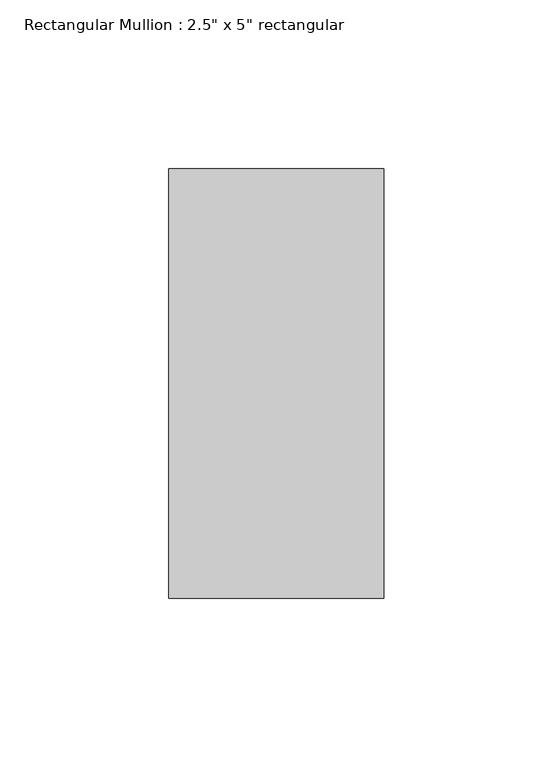
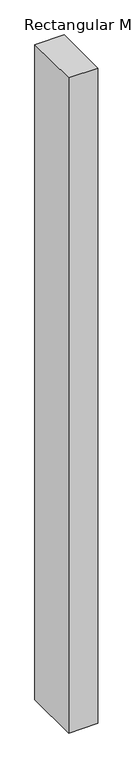
"""IFC4 building model written with IfcOpenShell, lengths in millimetres: member geometry."""

from ifc_helpers import new_model, si_unit, frame, origin, place, context, project, spatial, polyline, outline, extrude, source, transform, mapped, element, save


def member_90125dd4(model_context):
    return source(origin(), model_context, "Body", "SweptSolid", [
        extrude(outline(polyline([(0.0, 63.5), (0.0, -63.5), (-63.5, -63.5), (-63.5, 63.5), (0.0, 63.5)])), frame((0.0, 0.0, -1509.6020555), z_axis=(0.0, 0.0, 1.0), x_axis=(1.0, 0.0, 0.0)), (0.0, 0.0, 1.0), 1509.6020555),
    ])


if __name__ == "__main__":
    model = new_model("IFC4")
    model_context = context("Model", 3, world=origin())
    ifc_project = project(units=[si_unit("LENGTHUNIT", "METRE", prefix="MILLI")], contexts=[model_context])
    site = spatial("IfcSite", under=ifc_project)
    building = spatial("IfcBuilding", under=site)
    placement = place(None, origin())
    member_shape = member_90125dd4(model_context)
    element("IfcMember", 1, ObjectType="Rectangular Mullion : 2.5\" x 5\" rectangular", at=placement, inside=building, context=model_context, shape_type="MappedRepresentation", body=[
        mapped(member_shape, transform((0.0, 0.0, 0.0), x_axis=(1.0, 0.0, 0.0), y_axis=(0.0, 1.0, 0.0), z_axis=(0.0, 0.0, 1.0))),
    ])
    save(model, "model.ifc")

# Revit data of these elements
# Type "Rectangular Mullion : 2.5\" x 5\" rectangular"
#   built-in parameter 1007304 = 0.416667 (stored number, unit not read)
#   built-in parameter 1007301 = 0.104167 (stored number, unit not read)
#   built-in parameter 1007300 = 0.104167 (stored number, unit not read)
# Element 1 (IfcMember, "Rectangular Mullion : 2.5\" x 5\" rectangular")
#   Materials on its faces: "Aluminum"
# Materials
#   "Aluminum": class "Metal", colour RGB 247 247 247, transparency 0, Description = "Aluminum 6061", Cost = 0
